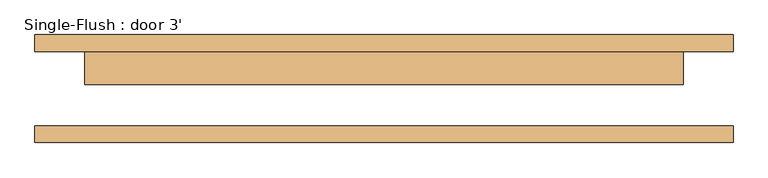
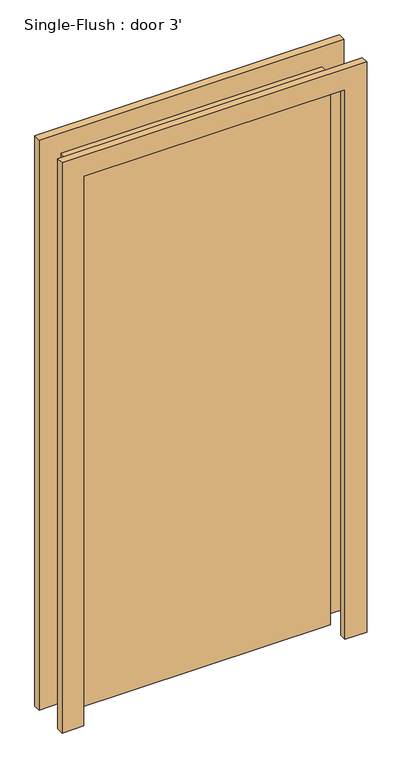
"""IFC4 building model written with IfcOpenShell, lengths in millimetres: door geometry, Single-Flush : door 3'."""

from ifc_helpers import new_model, si_unit, frame, origin, origin_with_axes, place, context, project, spatial, polyline, outline, extrude, source, transform, mapped, element, save


def single_flush_door_3_17d80c48(model_context):
    return source(origin(), model_context, "Body", "SweptSolid", [
        extrude(outline(polyline([(2108.2, -533.4), (0.0, -533.4), (0.0, -457.2), (2032.0, -457.2), (2032.0, 457.2), (0.0, 457.2), (0.0, 533.4), (2108.2, 533.4), (2108.2, -533.4)])), frame((0.0, 57.15, 0.0), z_axis=(0.0, 1.0, 0.0), x_axis=(0.0, 0.0, 1.0)), (0.0, 0.0, 1.0), 25.4),
        extrude(outline(polyline([(2108.2, 533.4), (2108.2, -533.4), (0.0, -533.4), (0.0, -457.2), (2032.0, -457.2), (2032.0, 457.2), (0.0, 457.2), (0.0, 533.4), (2108.2, 533.4)])), frame((0.0, -82.55, 0.0), z_axis=(0.0, 1.0, 0.0), x_axis=(0.0, 0.0, 1.0)), (0.0, 0.0, 1.0), 25.4),
        extrude(outline(polyline([(457.2, 6.35), (-457.2, 6.35), (-457.2, 57.15), (457.2, 57.15), (457.2, 6.35)])), origin_with_axes(), (0.0, 0.0, 1.0), 2032.0),
    ])


if __name__ == "__main__":
    model = new_model("IFC4")
    model_context = context("Model", 3, world=origin())
    ifc_project = project(units=[si_unit("LENGTHUNIT", "METRE", prefix="MILLI")], contexts=[model_context])
    site = spatial("IfcSite", under=ifc_project)
    building = spatial("IfcBuilding", under=site)
    placement = place(None, origin())
    single_flush_door_3_shape = single_flush_door_3_17d80c48(model_context)
    element("IfcDoor", 1, ObjectType="Single-Flush : door 3'", at=placement, inside=building, context=model_context, shape_type="MappedRepresentation", body=[
        mapped(single_flush_door_3_shape, transform((0.0, 0.0, 0.0), x_axis=(1.0, 0.0, 0.0), y_axis=(0.0, 1.0, 0.0), z_axis=(0.0, 0.0, 1.0))),
    ])
    save(model, "model.ifc")

# Revit data of these elements
# Type "Single-Flush : door 3'"
#   Type Mark = "9"
#   Construction Type Id = "MDOOR"
#   Assembly Code = "C1020"
#   Analytic Construction = "Metal"
#   Thickness = 0' - 2"
#   Heat Transfer Coefficient (U) = 0.651978 BTU/(h·ft²·°F)
#   Height = 6' - 8"
#   Trim Projection Ext = 0' - 1"
#   Trim Projection Int = 0' - 1"
#   Trim Width = 0' - 3"
#   Width = 3' - 0"
#   Define Thermal Properties by = 1
#   Door Material = Door - Panel
#   Frame Material = Door - Frame
#   Visual Light Transmittance = 0
#   Solar Heat Gain Coefficient = 0
#   Function = (empty or 0)
#   Wall Closure = (empty or 0)
# Element 1 (IfcDoor, "Single-Flush : door 3'")
#   Materials on its faces: "Door - Frame", "Door - Panel"
# Materials
#   "Door - Panel": class "Wood", colour RGB 210 159 95, transparency 0, Cost = 0
#   "Door - Frame": colour RGB 118 70 51, transparency 0, Cost = 0
